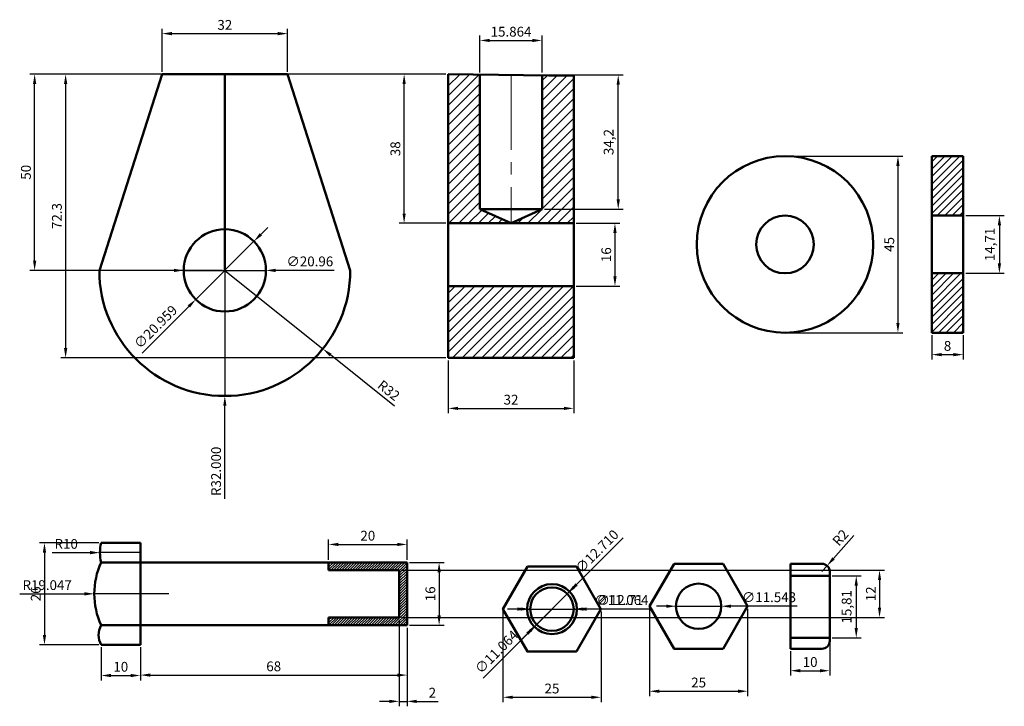
# Model space of a CAD drawing. Units: millimetres. Extents: x 1132 to 1696, y 1793 to 2376.
# Tile 1 of 4: x 1143 to 1394, y 1793 to 1968. Entities that reach past the tile are written whole.
import ezdxf

# ---------------------------------------------------------------- set-up
doc = ezdxf.new("R2010")
doc.units = ezdxf.units.MM
doc.linetypes.add('CENTER2', pattern=[28.575, 19.05, -3.175, 3.175, -3.175])
for name, color, linetype, lineweight in [('M-CNTR', 1, 'CENTER2', 18), ('M-DIMS', 2, 'Continuous', 25), ('M-HATC', 8, 'Continuous', 18), ('M-OUTL', 7, 'Continuous', 50)]:
    doc.layers.add(name, color=color, linetype=linetype, lineweight=lineweight)
doc.styles.get("Standard").update_dxf_attribs({"font": 'arial.ttf'})
doc.dimstyles.new('ISO-25', dxfattribs={"dimtxt": 2.5, "dimasz": 2.5, "dimexe": 1.25, "dimexo": 0.625, "dimtad": 1, "dimtxsty": 'Standard', "dimcen": 2.5, "dimadec": 0, "dimazin": 0, "dimtfac": 1, "dimtmove": 0, "dimatfit": 3, "dimfxl": 1, "dimarcsym": 0})

# ---------------------------------------------------------------- blocks, each defined once
blk = doc.blocks.new('*D15')
at = {"layer": 'Defpoints', "color": 0, "transparency": 16777216}
for p in [(1195.39, 1904.36), (1220.39, 1884.38)]:
    blk.add_point(p, dxfattribs=at)
at = {"layer": 'M-DIMS', "color": 0, "lineweight": -2, "transparency": 16777216}
for p, q in [((1195.39, 1904.36), (1220.39, 1884.38)), ((1238.63, 1869.8), (1222.34, 1882.82))]:
    blk.add_line(p, q, dxfattribs=at)
at = {"layer": 'M-DIMS', "color": 0, "transparency": 16777216}
blk.add_solid([(1222.6, 1883.14), (1222.08, 1882.49), (1220.39, 1884.38)], dxfattribs=at)
at = {"layer": 'M-DIMS', "color": 0, "transparency": 16777216, "insert": (1237.01, 1873.53), "char_height": 2.5, "attachment_point": 5, "rotation": 321.365}
blk.add_mtext('R32', dxfattribs=at)
blk = doc.blocks.new('*D16')
at = {"layer": 'Defpoints', "color": 0, "transparency": 16777216}
for p in [(1146.89, 1954.36), (1195.39, 1954.36), (1195.39, 1904.36)]:
    blk.add_point(p, dxfattribs=at)
at = {"layer": 'M-DIMS', "color": 0, "lineweight": -2, "transparency": 16777216}
for p, q in [((1194.77, 1954.36), (1145.64, 1954.36)), ((1146.89, 1906.86), (1146.89, 1951.86)), ((1194.77, 1904.36), (1145.64, 1904.36))]:
    blk.add_line(p, q, dxfattribs=at)
at = {"layer": 'M-DIMS', "color": 0, "transparency": 16777216}
for points in [[(1146.48, 1951.86), (1147.31, 1951.86), (1146.89, 1954.36)], [(1146.48, 1906.86), (1147.31, 1906.86), (1146.89, 1904.36)]]:
    blk.add_solid(points, dxfattribs=at)
at = {"layer": 'M-DIMS', "color": 0, "transparency": 16777216, "insert": (1144.99, 1929.36), "char_height": 2.5, "attachment_point": 5, "rotation": 90}
blk.add_mtext('50', dxfattribs=at)
blk = doc.blocks.new('*D17')
at = {"layer": 'Defpoints', "color": 0, "transparency": 16777216}
for p in [(1211.39, 1964.7), (1179.39, 1954.36), (1211.39, 1954.36)]:
    blk.add_point(p, dxfattribs=at)
at = {"layer": 'M-DIMS', "color": 0, "lineweight": -2, "transparency": 16777216}
for p, q in [((1179.39, 1954.98), (1179.39, 1965.95)), ((1181.89, 1964.7), (1208.89, 1964.7)), ((1211.39, 1954.98), (1211.39, 1965.95))]:
    blk.add_line(p, q, dxfattribs=at)
at = {"layer": 'M-DIMS', "color": 0, "transparency": 16777216}
for points in [[(1181.89, 1965.12), (1181.89, 1964.28), (1179.39, 1964.7)], [(1208.89, 1965.12), (1208.89, 1964.28), (1211.39, 1964.7)]]:
    blk.add_solid(points, dxfattribs=at)
at = {"layer": 'M-DIMS', "color": 0, "transparency": 16777216, "insert": (1195.39, 1966.6), "char_height": 2.5, "attachment_point": 5}
blk.add_mtext('32', dxfattribs=at)
blk = doc.blocks.new('*D18')
at = {"layer": 'Defpoints', "color": 0, "transparency": 16777216}
for p in [(1252.38, 1882.05), (1284.38, 1882.05), (1284.38, 1869.2)]:
    blk.add_point(p, dxfattribs=at)
at = {"layer": 'M-DIMS', "color": 0, "lineweight": -2, "transparency": 16777216}
for p, q in [((1252.38, 1881.43), (1252.38, 1867.95)), ((1284.38, 1881.43), (1284.38, 1867.95)), ((1254.88, 1869.2), (1281.88, 1869.2))]:
    blk.add_line(p, q, dxfattribs=at)
at = {"layer": 'M-DIMS', "color": 0, "transparency": 16777216}
for points in [[(1254.88, 1869.61), (1254.88, 1868.78), (1252.38, 1869.2)], [(1281.88, 1869.61), (1281.88, 1868.78), (1284.38, 1869.2)]]:
    blk.add_solid(points, dxfattribs=at)
at = {"layer": 'M-DIMS', "color": 0, "transparency": 16777216, "insert": (1268.38, 1871.1), "char_height": 2.5, "attachment_point": 5}
blk.add_mtext('32', dxfattribs=at)
blk = doc.blocks.new('*D19')
at = {"layer": 'Defpoints', "color": 0, "transparency": 16777216}
for p in [(1284.38, 1916.36), (1284.38, 1900.36), (1294.89, 1900.36)]:
    blk.add_point(p, dxfattribs=at)
at = {"layer": 'M-DIMS', "color": 0, "lineweight": -2, "transparency": 16777216}
for p, q in [((1285, 1916.36), (1296.14, 1916.36)), ((1294.89, 1913.86), (1294.89, 1902.86)), ((1285, 1900.36), (1296.14, 1900.36))]:
    blk.add_line(p, q, dxfattribs=at)
at = {"layer": 'M-DIMS', "color": 0, "transparency": 16777216}
for points in [[(1294.47, 1913.86), (1295.31, 1913.86), (1294.89, 1916.36)], [(1294.47, 1902.86), (1295.31, 1902.86), (1294.89, 1900.36)]]:
    blk.add_solid(points, dxfattribs=at)
at = {"layer": 'M-DIMS', "color": 0, "transparency": 16777216, "insert": (1292.99, 1908.36), "char_height": 2.5, "attachment_point": 5, "rotation": 90}
blk.add_mtext('16', dxfattribs=at)
blk = doc.blocks.new('*D20')
at = {"layer": 'Defpoints', "color": 0, "transparency": 16777216}
for p in [(1276.32, 1954.16), (1295.72, 1954.16), (1276.32, 1919.96)]:
    blk.add_point(p, dxfattribs=at)
at = {"layer": 'M-DIMS', "color": 0, "lineweight": -2, "transparency": 16777216}
for p, q in [((1276.94, 1954.16), (1296.97, 1954.16)), ((1295.72, 1922.46), (1295.72, 1951.66)), ((1276.94, 1919.96), (1296.97, 1919.96))]:
    blk.add_line(p, q, dxfattribs=at)
at = {"layer": 'M-DIMS', "color": 0, "transparency": 16777216}
for points in [[(1295.31, 1951.66), (1296.14, 1951.66), (1295.72, 1954.16)], [(1295.31, 1922.46), (1296.14, 1922.46), (1295.72, 1919.96)]]:
    blk.add_solid(points, dxfattribs=at)
at = {"layer": 'M-DIMS', "color": 0, "transparency": 16777216, "insert": (1293.6, 1937.06), "char_height": 2.5, "attachment_point": 5, "rotation": 90}
blk.add_mtext('34,2', dxfattribs=at)
blk = doc.blocks.new('*D21')
at = {"layer": 'Defpoints', "color": 0, "transparency": 16777216}
for p in [(1241.12, 1954.36), (1252.38, 1954.36), (1252.38, 1916.36)]:
    blk.add_point(p, dxfattribs=at)
at = {"layer": 'M-DIMS', "color": 0, "lineweight": -2, "transparency": 16777216}
for p, q in [((1251.75, 1954.36), (1239.87, 1954.36)), ((1241.12, 1918.86), (1241.12, 1951.86)), ((1251.75, 1916.36), (1239.87, 1916.36))]:
    blk.add_line(p, q, dxfattribs=at)
at = {"layer": 'M-DIMS', "color": 0, "transparency": 16777216}
for points in [[(1240.71, 1951.86), (1241.54, 1951.86), (1241.12, 1954.36)], [(1240.71, 1918.86), (1241.54, 1918.86), (1241.12, 1916.36)]]:
    blk.add_solid(points, dxfattribs=at)
at = {"layer": 'M-DIMS', "color": 0, "transparency": 16777216, "insert": (1239.22, 1935.36), "char_height": 2.5, "attachment_point": 5, "rotation": 90}
blk.add_mtext('38', dxfattribs=at)
blk = doc.blocks.new('*D22')
at = {"layer": 'Defpoints', "color": 0, "transparency": 16777216}
for p in [(1241.86, 1813.94), (1173.86, 1808.94), (1241.86, 1801.24)]:
    blk.add_point(p, dxfattribs=at)
at = {"layer": 'M-DIMS', "color": 0, "lineweight": -2, "transparency": 16777216}
for p, q in [((1241.86, 1813.32), (1241.86, 1799.99)), ((1173.86, 1808.32), (1173.86, 1799.99)), ((1176.36, 1801.24), (1239.36, 1801.24))]:
    blk.add_line(p, q, dxfattribs=at)
at = {"layer": 'M-DIMS', "color": 0, "transparency": 16777216}
for points in [[(1176.36, 1801.65), (1176.36, 1800.82), (1173.86, 1801.24)], [(1239.36, 1801.65), (1239.36, 1800.82), (1241.86, 1801.24)]]:
    blk.add_solid(points, dxfattribs=at)
at = {"layer": 'M-DIMS', "color": 0, "transparency": 16777216, "insert": (1207.86, 1803.14), "char_height": 2.5, "attachment_point": 5}
blk.add_mtext('68', dxfattribs=at)
blk = doc.blocks.new('*D23')
at = {"layer": 'Defpoints', "color": 0, "transparency": 16777216}
for p in [(1163.86, 1808.94), (1173.86, 1808.94), (1173.86, 1801.13)]:
    blk.add_point(p, dxfattribs=at)
at = {"layer": 'M-DIMS', "color": 0, "lineweight": -2, "transparency": 16777216}
for p, q in [((1163.86, 1808.32), (1163.86, 1799.88)), ((1173.86, 1808.32), (1173.86, 1799.88)), ((1166.36, 1801.13), (1171.36, 1801.13))]:
    blk.add_line(p, q, dxfattribs=at)
at = {"layer": 'M-DIMS', "color": 0, "transparency": 16777216}
for points in [[(1166.36, 1801.55), (1166.36, 1800.71), (1163.86, 1801.13)], [(1171.36, 1801.55), (1171.36, 1800.71), (1173.86, 1801.13)]]:
    blk.add_solid(points, dxfattribs=at)
at = {"layer": 'M-DIMS', "color": 0, "transparency": 16777216, "insert": (1168.86, 1803.03), "char_height": 2.5, "attachment_point": 5}
blk.add_mtext('10', dxfattribs=at)
blk = doc.blocks.new('*D24')
at = {"layer": 'Defpoints', "color": 0, "transparency": 16777216}
for p in [(1241.86, 1834.53), (1221.86, 1829.94), (1241.86, 1829.94)]:
    blk.add_point(p, dxfattribs=at)
at = {"layer": 'M-DIMS', "color": 0, "lineweight": -2, "transparency": 16777216}
for p, q in [((1221.86, 1830.57), (1221.86, 1835.78)), ((1241.86, 1830.57), (1241.86, 1835.78)), ((1224.36, 1834.53), (1239.36, 1834.53))]:
    blk.add_line(p, q, dxfattribs=at)
at = {"layer": 'M-DIMS', "color": 0, "transparency": 16777216}
for points in [[(1224.36, 1834.95), (1224.36, 1834.12), (1221.86, 1834.53)], [(1239.36, 1834.95), (1239.36, 1834.12), (1241.86, 1834.53)]]:
    blk.add_solid(points, dxfattribs=at)
at = {"layer": 'M-DIMS', "color": 0, "transparency": 16777216, "insert": (1231.86, 1836.43), "char_height": 2.5, "attachment_point": 5}
blk.add_mtext('20', dxfattribs=at)
blk = doc.blocks.new('*D25')
at = {"layer": 'Defpoints', "color": 0, "transparency": 16777216}
for p in [(1241.86, 1829.94), (1241.86, 1813.94), (1250.04, 1813.94)]:
    blk.add_point(p, dxfattribs=at)
at = {"layer": 'M-DIMS', "color": 0, "lineweight": -2, "transparency": 16777216}
for p, q in [((1242.49, 1829.94), (1251.29, 1829.94)), ((1250.04, 1827.44), (1250.04, 1816.44)), ((1242.49, 1813.94), (1251.29, 1813.94))]:
    blk.add_line(p, q, dxfattribs=at)
at = {"layer": 'M-DIMS', "color": 0, "transparency": 16777216}
for points in [[(1249.62, 1827.44), (1250.46, 1827.44), (1250.04, 1829.94)], [(1249.62, 1816.44), (1250.46, 1816.44), (1250.04, 1813.94)]]:
    blk.add_solid(points, dxfattribs=at)
at = {"layer": 'M-DIMS', "color": 0, "transparency": 16777216, "insert": (1248.14, 1821.94), "char_height": 2.5, "attachment_point": 5, "rotation": 90}
blk.add_mtext('16', dxfattribs=at)
blk = doc.blocks.new('*D26')
at = {"layer": 'Defpoints', "color": 0, "transparency": 16777216}
for p in [(1266.33, 1818.06), (1291.33, 1818.06), (1291.33, 1795.59)]:
    blk.add_point(p, dxfattribs=at)
at = {"layer": 'M-DIMS', "color": 0, "lineweight": -2, "transparency": 16777216}
for p, q in [((1266.33, 1817.44), (1266.33, 1794.34)), ((1291.33, 1817.44), (1291.33, 1794.34)), ((1268.83, 1795.59), (1288.83, 1795.59))]:
    blk.add_line(p, q, dxfattribs=at)
at = {"layer": 'M-DIMS', "color": 0, "transparency": 16777216}
for points in [[(1268.83, 1796), (1268.83, 1795.17), (1266.33, 1795.59)], [(1288.83, 1796), (1288.83, 1795.17), (1291.33, 1795.59)]]:
    blk.add_solid(points, dxfattribs=at)
at = {"layer": 'M-DIMS', "color": 0, "transparency": 16777216, "insert": (1278.83, 1797.49), "char_height": 2.5, "attachment_point": 5}
blk.add_mtext('25', dxfattribs=at)
blk = doc.blocks.new('*D27')
at = {"layer": 'Defpoints', "color": 0, "transparency": 16777216}
for p in [(1303.73, 1818.79), (1328.73, 1818.79), (1328.73, 1797.12)]:
    blk.add_point(p, dxfattribs=at)
at = {"layer": 'M-DIMS', "color": 0, "lineweight": -2, "transparency": 16777216}
for p, q in [((1303.73, 1818.16), (1303.73, 1795.87)), ((1328.73, 1818.16), (1328.73, 1795.87)), ((1306.23, 1797.12), (1326.23, 1797.12))]:
    blk.add_line(p, q, dxfattribs=at)
at = {"layer": 'M-DIMS', "color": 0, "transparency": 16777216}
for points in [[(1306.23, 1797.54), (1306.23, 1796.7), (1303.73, 1797.12)], [(1326.23, 1797.54), (1326.23, 1796.7), (1328.73, 1797.12)]]:
    blk.add_solid(points, dxfattribs=at)
at = {"layer": 'M-DIMS', "color": 0, "transparency": 16777216, "insert": (1316.23, 1799.02), "char_height": 2.5, "attachment_point": 5}
blk.add_mtext('25', dxfattribs=at)
blk = doc.blocks.new('*D28')
at = {"layer": 'Defpoints', "color": 0, "transparency": 16777216}
for p in [(1349.66, 1810.75), (1339.66, 1807.96), (1349.66, 1802.35)]:
    blk.add_point(p, dxfattribs=at)
at = {"layer": 'M-DIMS', "color": 0, "lineweight": -2, "transparency": 16777216}
for p, q in [((1349.66, 1810.12), (1349.66, 1801.1)), ((1339.66, 1807.34), (1339.66, 1801.1)), ((1342.16, 1802.35), (1347.16, 1802.35))]:
    blk.add_line(p, q, dxfattribs=at)
at = {"layer": 'M-DIMS', "color": 0, "transparency": 16777216}
for points in [[(1342.16, 1802.77), (1342.16, 1801.94), (1339.66, 1802.35)], [(1347.16, 1802.77), (1347.16, 1801.94), (1349.66, 1802.35)]]:
    blk.add_solid(points, dxfattribs=at)
at = {"layer": 'M-DIMS', "color": 0, "transparency": 16777216, "insert": (1344.66, 1804.25), "char_height": 2.5, "attachment_point": 5}
blk.add_mtext('10', dxfattribs=at)
blk = doc.blocks.new('*D29')
at = {"layer": 'Defpoints', "color": 0, "transparency": 16777216}
for p in [(1349.66, 1826.55), (1349.66, 1810.75), (1356.42, 1810.75)]:
    blk.add_point(p, dxfattribs=at)
at = {"layer": 'M-DIMS', "color": 0, "lineweight": -2, "transparency": 16777216}
for p, q in [((1350.29, 1826.55), (1357.67, 1826.55)), ((1356.42, 1824.05), (1356.42, 1813.25)), ((1350.29, 1810.75), (1357.67, 1810.75))]:
    blk.add_line(p, q, dxfattribs=at)
at = {"layer": 'M-DIMS', "color": 0, "transparency": 16777216}
for points in [[(1356.01, 1824.05), (1356.84, 1824.05), (1356.42, 1826.55)], [(1356.01, 1813.25), (1356.84, 1813.25), (1356.42, 1810.75)]]:
    blk.add_solid(points, dxfattribs=at)
at = {"layer": 'M-DIMS', "color": 0, "transparency": 16777216, "insert": (1354.29, 1818.65), "char_height": 2.5, "attachment_point": 5, "rotation": 90}
blk.add_mtext('15,81', dxfattribs=at)
blk = doc.blocks.new('*D30')
at = {"layer": 'Defpoints', "color": 0, "transparency": 16777216}
for p in [(1338.27, 1933.48), (1338.27, 1888.48), (1367.06, 1888.48)]:
    blk.add_point(p, dxfattribs=at)
at = {"layer": 'M-DIMS', "color": 0, "lineweight": -2, "transparency": 16777216}
for p, q in [((1338.9, 1933.48), (1368.31, 1933.48)), ((1367.06, 1930.98), (1367.06, 1890.98)), ((1338.9, 1888.48), (1368.31, 1888.48))]:
    blk.add_line(p, q, dxfattribs=at)
at = {"layer": 'M-DIMS', "color": 0, "transparency": 16777216}
for points in [[(1366.64, 1930.98), (1367.47, 1930.98), (1367.06, 1933.48)], [(1366.64, 1890.98), (1367.47, 1890.98), (1367.06, 1888.48)]]:
    blk.add_solid(points, dxfattribs=at)
at = {"layer": 'M-DIMS', "color": 0, "transparency": 16777216, "insert": (1365.16, 1910.98), "char_height": 2.5, "attachment_point": 5, "rotation": 90}
blk.add_mtext('45', dxfattribs=at)
blk = doc.blocks.new('*D31')
at = {"layer": 'Defpoints', "color": 0, "transparency": 16777216}
for p in [(1375.71, 1888.48), (1383.71, 1888.48), (1383.71, 1882.89)]:
    blk.add_point(p, dxfattribs=at)
at = {"layer": 'M-DIMS', "color": 0, "lineweight": -2, "transparency": 16777216}
for p, q in [((1375.71, 1887.85), (1375.71, 1881.64)), ((1383.71, 1887.85), (1383.71, 1881.64)), ((1378.21, 1882.89), (1381.21, 1882.89))]:
    blk.add_line(p, q, dxfattribs=at)
at = {"layer": 'M-DIMS', "color": 0, "transparency": 16777216}
for points in [[(1378.21, 1883.31), (1378.21, 1882.48), (1375.71, 1882.89)], [(1381.21, 1883.31), (1381.21, 1882.48), (1383.71, 1882.89)]]:
    blk.add_solid(points, dxfattribs=at)
at = {"layer": 'M-DIMS', "color": 0, "transparency": 16777216, "insert": (1379.71, 1884.8), "char_height": 2.5, "attachment_point": 5}
blk.add_mtext('8', dxfattribs=at)
blk = doc.blocks.new('*D32')
at = {"layer": 'Defpoints', "color": 0, "transparency": 16777216}
for p in [(1383.71, 1918.33), (1383.71, 1903.62), (1392.93, 1903.62)]:
    blk.add_point(p, dxfattribs=at)
at = {"layer": 'M-DIMS', "color": 0, "lineweight": -2, "transparency": 16777216}
for p, q in [((1384.33, 1918.33), (1394.18, 1918.33)), ((1392.93, 1915.83), (1392.93, 1906.12)), ((1384.33, 1903.62), (1394.18, 1903.62))]:
    blk.add_line(p, q, dxfattribs=at)
at = {"layer": 'M-DIMS', "color": 0, "transparency": 16777216}
for points in [[(1392.52, 1915.83), (1393.35, 1915.83), (1392.93, 1918.33)], [(1392.52, 1906.12), (1393.35, 1906.12), (1392.93, 1903.62)]]:
    blk.add_solid(points, dxfattribs=at)
at = {"layer": 'M-DIMS', "color": 0, "transparency": 16777216, "insert": (1390.81, 1910.98), "char_height": 2.5, "attachment_point": 5, "rotation": 90}
blk.add_mtext('14,71', dxfattribs=at)
blk = doc.blocks.new('*D39')
at = {"layer": 'Defpoints', "color": 0, "transparency": 16777216}
for p in [(1276.32, 1962.96), (1260.45, 1954.16), (1276.32, 1954.16)]:
    blk.add_point(p, dxfattribs=at)
at = {"layer": 'M-DIMS', "color": 0, "lineweight": -2, "transparency": 16777216}
for p, q in [((1260.45, 1954.78), (1260.45, 1964.21)), ((1276.32, 1954.78), (1276.32, 1964.21)), ((1262.95, 1962.96), (1273.82, 1962.96))]:
    blk.add_line(p, q, dxfattribs=at)
at = {"layer": 'M-DIMS', "color": 0, "transparency": 16777216}
for points in [[(1262.95, 1963.37), (1262.95, 1962.54), (1260.45, 1962.96)], [(1273.82, 1963.37), (1273.82, 1962.54), (1276.32, 1962.96)]]:
    blk.add_solid(points, dxfattribs=at)
at = {"layer": 'M-DIMS', "color": 0, "transparency": 16777216, "insert": (1268.39, 1964.86), "char_height": 2.5, "attachment_point": 5}
blk.add_mtext('15.864', dxfattribs=at)
blk = doc.blocks.new('*D40')
at = {"layer": 'Defpoints', "color": 0, "transparency": 16777216}
for p in [(1252.38, 1954.36), (1154.79, 1882.05), (1252.38, 1882.05)]:
    blk.add_point(p, dxfattribs=at)
at = {"layer": 'M-DIMS', "color": 0, "lineweight": -2, "transparency": 16777216}
for p, q in [((1251.75, 1954.36), (1153.54, 1954.36)), ((1154.79, 1951.86), (1154.79, 1884.55)), ((1251.75, 1882.05), (1153.54, 1882.05))]:
    blk.add_line(p, q, dxfattribs=at)
at = {"layer": 'M-DIMS', "color": 0, "transparency": 16777216}
for points in [[(1154.38, 1951.86), (1155.21, 1951.86), (1154.79, 1954.36)], [(1154.38, 1884.55), (1155.21, 1884.55), (1154.79, 1882.05)]]:
    blk.add_solid(points, dxfattribs=at)
at = {"layer": 'M-DIMS', "color": 0, "transparency": 16777216, "insert": (1152.89, 1918.21), "char_height": 2.5, "attachment_point": 5, "rotation": 90}
blk.add_mtext('72.3', dxfattribs=at)
blk = doc.blocks.new('*D46')
at = {"layer": 'Defpoints', "color": 0, "transparency": 16777216}
for p in [(1163.86, 1834.94), (1149.4, 1808.94), (1163.86, 1808.94)]:
    blk.add_point(p, dxfattribs=at)
at = {"layer": 'M-DIMS', "color": 0, "lineweight": -2, "transparency": 16777216}
for p, q in [((1163.24, 1834.94), (1148.15, 1834.94)), ((1149.4, 1832.44), (1149.4, 1811.44)), ((1163.24, 1808.94), (1148.15, 1808.94))]:
    blk.add_line(p, q, dxfattribs=at)
at = {"layer": 'M-DIMS', "color": 0, "transparency": 16777216}
for points in [[(1148.98, 1832.44), (1149.82, 1832.44), (1149.4, 1834.94)], [(1148.98, 1811.44), (1149.82, 1811.44), (1149.4, 1808.94)]]:
    blk.add_solid(points, dxfattribs=at)
at = {"layer": 'M-DIMS', "color": 0, "transparency": 16777216, "insert": (1147.5, 1821.94), "char_height": 2.5, "attachment_point": 5, "rotation": 90}
blk.add_mtext('26', dxfattribs=at)
blk = doc.blocks.new('*D47')
at = {"layer": 'Defpoints', "color": 0, "transparency": 16777216}
for p in [(1239.86, 1827.94), (1239.86, 1815.94), (1362.36, 1815.94)]:
    blk.add_point(p, dxfattribs=at)
at = {"layer": 'M-DIMS', "color": 0, "lineweight": -2, "transparency": 16777216}
for p, q in [((1240.49, 1827.94), (1363.61, 1827.94)), ((1362.36, 1825.44), (1362.36, 1818.44)), ((1240.49, 1815.94), (1363.61, 1815.94))]:
    blk.add_line(p, q, dxfattribs=at)
at = {"layer": 'M-DIMS', "color": 0, "transparency": 16777216}
for points in [[(1361.95, 1825.44), (1362.78, 1825.44), (1362.36, 1827.94)], [(1361.95, 1818.44), (1362.78, 1818.44), (1362.36, 1815.94)]]:
    blk.add_solid(points, dxfattribs=at)
at = {"layer": 'M-DIMS', "color": 0, "transparency": 16777216, "insert": (1360.48, 1821.94), "char_height": 2.5, "attachment_point": 5, "rotation": 90}
blk.add_mtext('12', dxfattribs=at)
blk = doc.blocks.new('*D48')
at = {"layer": 'Defpoints', "color": 0, "transparency": 16777216}
for p in [(1239.86, 1815.94), (1241.86, 1813.94), (1241.86, 1794.54)]:
    blk.add_point(p, dxfattribs=at)
at = {"layer": 'M-DIMS', "color": 0, "lineweight": -2, "transparency": 16777216}
for p, q in [((1239.86, 1815.32), (1239.86, 1793.29)), ((1241.86, 1813.32), (1241.86, 1793.29)), ((1237.36, 1794.54), (1234.86, 1794.54)), ((1239.86, 1794.54), (1241.86, 1794.54)), ((1244.36, 1794.54), (1249.77, 1794.54))]:
    blk.add_line(p, q, dxfattribs=at)
at = {"layer": 'M-DIMS', "color": 0, "transparency": 16777216}
for points in [[(1237.36, 1794.95), (1237.36, 1794.12), (1239.86, 1794.54)], [(1244.36, 1794.95), (1244.36, 1794.12), (1241.86, 1794.54)]]:
    blk.add_solid(points, dxfattribs=at)
at = {"layer": 'M-DIMS', "color": 0, "transparency": 16777216, "insert": (1248.32, 1796.42), "char_height": 2.5, "attachment_point": 5}
blk.add_mtext('2', dxfattribs=at)
blk = doc.blocks.new('*D50')
at = {"layer": 'Defpoints', "color": 0, "transparency": 16777216}
for p in [(1184.91, 1904.36), (1205.87, 1904.36)]:
    blk.add_point(p, dxfattribs=at)
at = {"layer": 'M-DIMS', "color": 0, "lineweight": -2, "transparency": 16777216}
for p, q in [((1182.41, 1904.36), (1179.91, 1904.36)), ((1184.91, 1904.36), (1205.87, 1904.36)), ((1223.28, 1904.36), (1208.37, 1904.36))]:
    blk.add_line(p, q, dxfattribs=at)
at = {"layer": 'M-DIMS', "color": 0, "transparency": 16777216}
for points in [[(1182.41, 1904.78), (1182.41, 1903.94), (1184.91, 1904.36)], [(1208.37, 1904.77), (1208.37, 1903.94), (1205.87, 1904.36)]]:
    blk.add_solid(points, dxfattribs=at)
at = {"layer": 'M-DIMS', "color": 0, "transparency": 16777216, "insert": (1217.08, 1906.33), "char_height": 2.5, "attachment_point": 5, "rotation": 359.9985}
blk.add_mtext('∅20.96', dxfattribs=at)
blk = doc.blocks.new('*D54')
at = {"layer": 'Defpoints', "color": 0, "transparency": 16777216}
for p in [(1162.1, 1821.94), (1181.15, 1821.94)]:
    blk.add_point(p, dxfattribs=at)
at = {"layer": 'M-DIMS', "color": 0, "lineweight": -2, "transparency": 16777216}
for p, q in [((1143.08, 1821.94), (1159.6, 1821.94)), ((1181.15, 1821.94), (1162.1, 1821.94))]:
    blk.add_line(p, q, dxfattribs=at)
at = {"layer": 'M-DIMS', "color": 0, "transparency": 16777216}
blk.add_solid([(1159.6, 1822.36), (1159.6, 1821.53), (1162.1, 1821.94)], dxfattribs=at)
at = {"layer": 'M-DIMS', "color": 0, "transparency": 16777216, "insert": (1150.09, 1823.84), "char_height": 2.5, "attachment_point": 5, "rotation": 0.0015}
blk.add_mtext('R19.047', dxfattribs=at)
blk = doc.blocks.new('*D55')
at = {"layer": 'Defpoints', "color": 0, "transparency": 16777216}
for p in [(1163.55, 1832.44), (1173.55, 1832.44)]:
    blk.add_point(p, dxfattribs=at)
at = {"layer": 'M-DIMS', "color": 0, "lineweight": -2, "transparency": 16777216}
for p, q in [((1151.33, 1832.44), (1161.05, 1832.44)), ((1173.55, 1832.44), (1163.55, 1832.44))]:
    blk.add_line(p, q, dxfattribs=at)
at = {"layer": 'M-DIMS', "color": 0, "transparency": 16777216}
blk.add_solid([(1161.05, 1832.86), (1161.05, 1832.03), (1163.55, 1832.44)], dxfattribs=at)
at = {"layer": 'M-DIMS', "color": 0, "transparency": 16777216, "insert": (1154.94, 1834.34), "char_height": 2.5, "attachment_point": 5, "rotation": 0.0028}
blk.add_mtext('R10', dxfattribs=at)
blk = doc.blocks.new('*D56')
at = {"layer": 'Defpoints', "color": 0, "transparency": 16777216}
for p in [(1272.47, 1818.06), (1285.18, 1818.06)]:
    blk.add_point(p, dxfattribs=at)
at = {"layer": 'M-DIMS', "color": 0, "lineweight": -2, "transparency": 16777216}
for p, q in [((1269.97, 1818.06), (1267.47, 1818.06)), ((1272.47, 1818.06), (1285.18, 1818.06)), ((1302.11, 1818.06), (1287.68, 1818.06))]:
    blk.add_line(p, q, dxfattribs=at)
at = {"layer": 'M-DIMS', "color": 0, "transparency": 16777216}
for points in [[(1269.97, 1818.48), (1269.97, 1817.65), (1272.47, 1818.06)], [(1287.68, 1818.48), (1287.68, 1817.64), (1285.18, 1818.06)]]:
    blk.add_solid(points, dxfattribs=at)
at = {"layer": 'M-DIMS', "color": 0, "transparency": 16777216, "insert": (1296.15, 1820.03), "char_height": 2.5, "attachment_point": 5, "rotation": 359.9964}
blk.add_mtext('∅12.71', dxfattribs=at)
blk = doc.blocks.new('*D57')
at = {"layer": 'Defpoints', "color": 0, "transparency": 16777216}
for p in [(1273.3, 1818.06), (1284.36, 1818.06)]:
    blk.add_point(p, dxfattribs=at)
at = {"layer": 'M-DIMS', "color": 0, "lineweight": -2, "transparency": 16777216}
for p, q in [((1270.8, 1818.06), (1268.3, 1818.06)), ((1273.3, 1818.06), (1284.36, 1818.06)), ((1303.7, 1818.06), (1286.86, 1818.06))]:
    blk.add_line(p, q, dxfattribs=at)
at = {"layer": 'M-DIMS', "color": 0, "transparency": 16777216}
for points in [[(1270.8, 1818.48), (1270.8, 1817.65), (1273.3, 1818.06)], [(1286.86, 1818.48), (1286.86, 1817.64), (1284.36, 1818.06)]]:
    blk.add_solid(points, dxfattribs=at)
at = {"layer": 'M-DIMS', "color": 0, "transparency": 16777216, "insert": (1296.53, 1820.03), "char_height": 2.5, "attachment_point": 5, "rotation": 359.9959}
blk.add_mtext('∅11.064', dxfattribs=at)
blk = doc.blocks.new('*D58')
at = {"layer": 'Defpoints', "color": 0, "transparency": 16777216}
for p in [(1310.46, 1818.79), (1322, 1818.79)]:
    blk.add_point(p, dxfattribs=at)
at = {"layer": 'M-DIMS', "color": 0, "lineweight": -2, "transparency": 16777216}
for p, q in [((1307.96, 1818.79), (1305.46, 1818.79)), ((1310.46, 1818.79), (1322, 1818.79)), ((1341.35, 1818.78), (1324.5, 1818.79))]:
    blk.add_line(p, q, dxfattribs=at)
at = {"layer": 'M-DIMS', "color": 0, "transparency": 16777216}
for points in [[(1307.96, 1819.2), (1307.96, 1818.37), (1310.46, 1818.79)], [(1324.5, 1819.2), (1324.5, 1818.37), (1322, 1818.79)]]:
    blk.add_solid(points, dxfattribs=at)
at = {"layer": 'M-DIMS', "color": 0, "transparency": 16777216, "insert": (1334.17, 1820.76), "char_height": 2.5, "attachment_point": 5, "rotation": 359.9969}
blk.add_mtext('∅11.543', dxfattribs=at)
blk = doc.blocks.new('*D59')
at = {"layer": 'Defpoints', "color": 0, "transparency": 16777216}
for p in [(1348.99, 1829.11), (1347.66, 1827.61)]:
    blk.add_point(p, dxfattribs=at)
at = {"layer": 'M-DIMS', "color": 0, "lineweight": -2, "transparency": 16777216}
for p, q in [((1355.79, 1836.79), (1350.65, 1830.98)), ((1347.66, 1827.61), (1348.99, 1829.11))]:
    blk.add_line(p, q, dxfattribs=at)
at = {"layer": 'M-DIMS', "color": 0, "transparency": 16777216}
blk.add_solid([(1350.33, 1831.26), (1350.96, 1830.7), (1348.99, 1829.11)], dxfattribs=at)
at = {"layer": 'M-DIMS', "color": 0, "transparency": 16777216, "insert": (1352.64, 1836.07), "char_height": 2.5, "attachment_point": 5, "rotation": 48.4719}
blk.add_mtext('R2', dxfattribs=at)
blk = doc.blocks.new('*D86')
at = {"layer": 'Defpoints', "color": 0, "transparency": 16777216}
for p in [(1202.81, 1911.77), (1187.98, 1896.95)]:
    blk.add_point(p, dxfattribs=at)
at = {"layer": 'M-DIMS', "color": 0, "lineweight": -2, "transparency": 16777216}
for p, q in [((1204.57, 1913.53), (1206.34, 1915.3)), ((1202.81, 1911.77), (1187.98, 1896.95)), ((1174.29, 1883.27), (1186.21, 1895.18))]:
    blk.add_line(p, q, dxfattribs=at)
at = {"layer": 'M-DIMS', "color": 0, "transparency": 16777216}
for points in [[(1204.28, 1913.83), (1204.87, 1913.24), (1202.81, 1911.77)], [(1185.92, 1895.48), (1186.51, 1894.89), (1187.98, 1896.95)]]:
    blk.add_solid(points, dxfattribs=at)
at = {"layer": 'M-DIMS', "color": 0, "transparency": 16777216, "insert": (1177.97, 1889.74), "char_height": 2.5, "attachment_point": 5, "rotation": 44.9813}
blk.add_mtext('∅20.959', dxfattribs=at)
blk = doc.blocks.new('*D87')
at = {"layer": 'Defpoints', "color": 0, "transparency": 16777216}
for p in [(1195.39, 1904.36), (1195.39, 1872.36)]:
    blk.add_point(p, dxfattribs=at)
at = {"layer": 'M-DIMS', "color": 0, "lineweight": -2, "transparency": 16777216}
for p, q in [((1195.39, 1904.36), (1195.39, 1872.36)), ((1195.39, 1846.15), (1195.39, 1869.86))]:
    blk.add_line(p, q, dxfattribs=at)
at = {"layer": 'M-DIMS', "color": 0, "transparency": 16777216}
blk.add_solid([(1194.98, 1869.86), (1195.81, 1869.86), (1195.39, 1872.36)], dxfattribs=at)
at = {"layer": 'M-DIMS', "color": 0, "transparency": 16777216, "insert": (1193.49, 1853.16), "char_height": 2.5, "attachment_point": 5, "rotation": 89.9998}
blk.add_mtext('R32.000', dxfattribs=at)
blk = doc.blocks.new('*D88')
at = {"layer": 'Defpoints', "color": 0, "transparency": 16777216}
for p in [(1283.32, 1822.55), (1274.33, 1813.57)]:
    blk.add_point(p, dxfattribs=at)
at = {"layer": 'M-DIMS', "color": 0, "lineweight": -2, "transparency": 16777216}
for p, q in [((1297, 1836.23), (1285.09, 1824.32)), ((1274.33, 1813.57), (1283.32, 1822.55)), ((1272.57, 1811.8), (1270.8, 1810.03))]:
    blk.add_line(p, q, dxfattribs=at)
at = {"layer": 'M-DIMS', "color": 0, "transparency": 16777216}
for points in [[(1284.8, 1824.62), (1285.39, 1824.03), (1283.32, 1822.55)], [(1272.27, 1812.1), (1272.86, 1811.51), (1274.33, 1813.57)]]:
    blk.add_solid(points, dxfattribs=at)
at = {"layer": 'M-DIMS', "color": 0, "transparency": 16777216, "insert": (1290.54, 1832.55), "char_height": 2.5, "attachment_point": 5, "rotation": 44.983}
blk.add_mtext('∅12.710', dxfattribs=at)
blk = doc.blocks.new('*D89')
at = {"layer": 'Defpoints', "color": 0, "transparency": 16777216}
for p in [(1282.74, 1821.97), (1274.92, 1814.15)]:
    blk.add_point(p, dxfattribs=at)
at = {"layer": 'M-DIMS', "color": 0, "lineweight": -2, "transparency": 16777216}
for p, q in [((1284.51, 1823.74), (1286.27, 1825.51)), ((1282.74, 1821.97), (1274.92, 1814.15)), ((1261.25, 1800.47), (1273.15, 1812.38))]:
    blk.add_line(p, q, dxfattribs=at)
at = {"layer": 'M-DIMS', "color": 0, "transparency": 16777216}
for points in [[(1284.21, 1824.04), (1284.8, 1823.45), (1282.74, 1821.97)], [(1272.86, 1812.67), (1273.45, 1812.09), (1274.92, 1814.15)]]:
    blk.add_solid(points, dxfattribs=at)
at = {"layer": 'M-DIMS', "color": 0, "transparency": 16777216, "insert": (1264.92, 1806.93), "char_height": 2.5, "attachment_point": 5, "rotation": 45.0195}
blk.add_mtext('∅11.064', dxfattribs=at)

msp = doc.modelspace()

# ---------------------------------------------------------------- hatches: boundary and pattern name
at = {"layer": 'M-HATC'}
h = msp.add_hatch(dxfattribs=at)
h.set_pattern_fill('ANSI31', color=256, scale=0.56)
h.paths.add_polyline_path([(1284.3772, 1953.9602), (1276.3177, 1954.0604), (1276.3177, 1919.9602), (1268.3772, 1916.3583), (1284.3772, 1916.3583)])
h.paths.add_polyline_path([(1260.4541, 1919.9602), (1260.4541, 1954.2578), (1252.3772, 1954.3583), (1252.3772, 1916.3583), (1268.3772, 1916.3583)])
h.paths.add_polyline_path([(1284.3772, 1900.3583), (1252.3772, 1900.3583), (1252.3772, 1882.0542), (1284.3772, 1882.0542)])
h = msp.add_hatch(dxfattribs=at)
h.set_pattern_fill('ANSI31', color=256, scale=0.42)
h.paths.add_polyline_path([(1383.7067, 1933.4789), (1375.7067, 1933.4789), (1375.7067, 1918.3333), (1383.7067, 1918.3333)])
h.paths.add_polyline_path([(1383.7067, 1903.6246), (1375.7067, 1903.6246), (1375.7067, 1888.4789), (1383.7067, 1888.4789)])
h = msp.add_hatch(dxfattribs=at)
h.set_pattern_fill('ANSI31', color=256, scale=0.15)
h.paths.add_polyline_path([(1241.8628, 1829.9425), (1221.8628, 1829.9425), (1221.8628, 1827.9425), (1239.8628, 1827.9425), (1239.8628, 1815.9425), (1221.8628, 1815.9425), (1221.8628, 1813.9425), (1241.8628, 1813.9425)])

# ---------------------------------------------------------------- linework, layer by layer
at = {"layer": 'M-CNTR'}
msp.add_line((1268.3772, 1954.1592), (1268.3772, 1916.3583), dxfattribs=at)
at = {"layer": 'M-OUTL'}
for p, q in [((1163.3931, 1904.3583), (1179.3931, 1954.3583)), ((1179.3931, 1954.3583), (1211.3931, 1954.3583)), ((1195.3931, 1954.3583), (1195.3931, 1904.3583)), ((1211.3931, 1954.3583), (1227.3931, 1904.3583)), ((1252.3772, 1954.3583), (1252.3772, 1882.0542)), ((1284.3772, 1953.9602), (1252.3772, 1954.3583)), ((1252.3772, 1954.3583), (1252.3772, 1916.3583)), ((1260.4541, 1954.1592), (1260.4541, 1919.9602)), ((1276.3177, 1954.1592), (1276.3177, 1919.9602)), ((1284.3772, 1882.0542), (1284.3772, 1953.9602)), ((1284.3772, 1953.9602), (1284.3772, 1919.9602)), ((1375.7067, 1933.4789), (1375.7067, 1888.4789)), ((1383.7067, 1933.4789), (1375.7067, 1933.4789)), ((1383.7067, 1888.4789), (1383.7067, 1933.4789)), ((1276.3177, 1919.9602), (1260.4541, 1919.9602)), ((1260.4541, 1919.9602), (1268.3772, 1916.3583)), ((1268.3772, 1916.3583), (1276.3177, 1919.9602)), ((1252.3772, 1916.3583), (1284.3772, 1916.3583)), ((1375.7067, 1918.3333), (1383.7067, 1918.3333)), ((1375.7067, 1903.6246), (1383.7067, 1903.6246)), ((1284.3772, 1900.3583), (1252.3772, 1900.3583)), ((1375.7067, 1888.4789), (1383.7067, 1888.4789)), ((1252.3772, 1882.0542), (1284.3772, 1882.0542)), ((1173.8628, 1834.9425), (1163.8628, 1834.9425)), ((1173.8628, 1829.9425), (1173.8628, 1834.9425)), ((1173.8628, 1829.9425), (1163.8628, 1829.9425)), ((1173.8628, 1829.9425), (1241.8628, 1829.9425)), ((1173.8628, 1813.9425), (1173.8628, 1829.9425)), ((1241.8628, 1829.9425), (1221.8628, 1829.9425)), ((1221.8628, 1829.9425), (1221.8628, 1827.9425)), ((1241.8628, 1829.9425), (1241.8628, 1813.9425)), ((1339.662, 1829.6116), (1339.662, 1807.961)), ((1339.662, 1829.6116), (1347.662, 1829.6116)), ((1221.8628, 1827.9425), (1239.8628, 1827.9425)), ((1239.8628, 1827.9425), (1239.8628, 1815.9425)), ((1339.662, 1826.5548), (1349.662, 1826.5548)), ((1349.662, 1809.961), (1349.662, 1827.6116)), ((1239.8628, 1815.9425), (1221.8628, 1815.9425)), ((1221.8628, 1815.9425), (1221.8628, 1813.9425)), ((1173.8628, 1813.9425), (1163.8628, 1813.9425)), ((1241.8628, 1813.9425), (1173.8628, 1813.9425)), ((1173.8628, 1808.9425), (1173.8628, 1813.9425)), ((1339.662, 1810.7467), (1349.662, 1810.7467)), ((1163.8628, 1808.9425), (1173.8628, 1808.9425)), ((1339.662, 1807.961), (1347.662, 1807.961))]:
    msp.add_line(p, q, dxfattribs=at)
for points in [[(1272.5787, 1828.8867), (1266.3287, 1818.0614), (1272.5787, 1807.2361), (1285.0787, 1807.2361), (1291.3287, 1818.0614), (1285.0787, 1828.8867)], [(1309.9765, 1829.6116), (1303.7265, 1818.7863), (1309.9765, 1807.961), (1322.4765, 1807.961), (1328.7265, 1818.7863), (1322.4765, 1829.6116)]]:
    msp.add_lwpolyline(points, close=True, dxfattribs=at)
for centre, radius in [((1338.2703, 1910.9789), 22.5), ((1338.2703, 1910.9789), 7.3543), ((1195.3931, 1904.3583), 10.4797), ((1278.8287, 1818.0614), 6.3549), ((1278.8287, 1818.0614), 5.5322), ((1316.2265, 1818.7863), 5.7714)]:
    msp.add_circle(centre, radius, dxfattribs=at)
for centre, radius, start, end in [((1195.3931, 1904.3583), 32, 180, 0), ((1173.5452, 1832.4425), 10, 165.522488, 194.477512), ((1181.1487, 1821.9425), 19.0474, 155.165061, 204.834939), ((1347.662, 1827.6116), 2, 360, 90), ((1168.1929, 1811.4425), 5, 150, 210), ((1347.662, 1809.961), 2, 270, 360)]:
    msp.add_arc(centre, radius, start, end, dxfattribs=at)

# ---------------------------------------------------------------- dimensions: what is measured, and where the dimension line sits
at = {"layer": 'M-DIMS'}
for base, p1, p2, override, picture, middle in [((1211.3931, 1964.7008), (1179.3931, 1954.3583), (1211.3931, 1954.3583), {"dimclrd": 0, "dimclre": 0, "dimclrt": 0}, '*D17', (1195.3931, 1966.6031)), ((1276.3177, 1962.9583), (1260.4541, 1954.1592), (1276.3177, 1954.1592), {"dimdec": 3, "dimlfac": 1, "dimrnd": 0, "dimzin": 0, "dimdsep": 46, "dimlunit": 2}, '*D39', (1268.3859, 1964.8597)), ((1383.7067, 1882.8936), (1375.7067, 1888.4789), (1383.7067, 1888.4789), {"dimclrd": 0, "dimclre": 0, "dimclrt": 0}, '*D31', (1379.7067, 1884.795)), ((1284.3772, 1869.1954), (1252.3772, 1882.0542), (1284.3772, 1882.0542), {"dimclrd": 0, "dimclre": 0, "dimclrt": 0}, '*D18', (1268.3772, 1871.0977)), ((1241.8628, 1834.5326), (1221.8628, 1829.9425), (1241.8628, 1829.9425), {"dimclrd": 0, "dimclre": 0, "dimclrt": 0}, '*D24', (1231.8628, 1836.434)), ((1291.3287, 1795.5869), (1266.3287, 1818.0614), (1291.3287, 1818.0614), {"dimclrd": 0, "dimclre": 0, "dimclrt": 0}, '*D26', (1278.8287, 1797.4884)), ((1328.7265, 1797.1187), (1303.7265, 1818.7863), (1328.7265, 1818.7863), {"dimclrd": 0, "dimclre": 0, "dimclrt": 0}, '*D27', (1316.2265, 1799.0202)), ((1241.8628, 1794.5361), (1239.8628, 1815.9425), (1241.8628, 1813.9425), {"dimdec": 0, "dimlfac": 1, "dimrnd": 0, "dimzin": 0, "dimdsep": 46, "dimlunit": 2}, '*D48', (1248.3157, 1796.4162)), ((1241.8628, 1801.2366), (1173.8628, 1808.9425), (1241.8628, 1813.9425), {"dimclrd": 0, "dimclre": 0, "dimclrt": 0}, '*D22', (1207.8628, 1803.138)), ((1349.662, 1802.3525), (1339.662, 1807.961), (1349.662, 1810.7467), {"dimclrd": 0, "dimclre": 0, "dimclrt": 0}, '*D28', (1344.662, 1804.2539)), ((1173.8628, 1801.1285), (1163.8628, 1808.9425), (1173.8628, 1808.9425), {"dimclrd": 0, "dimclre": 0, "dimclrt": 0}, '*D23', (1168.8628, 1803.03))]:
    dim = msp.add_linear_dim(base=base, p1=p1, p2=p2, dimstyle='ISO-25', override=override, dxfattribs=at)
    dim.commit()
    dim.dimension.update_dxf_attribs({"geometry": picture, "text_midpoint": middle})
for base, p1, p2, override, picture, middle in [((1146.894, 1954.3583), (1195.3931, 1904.3583), (1195.3931, 1954.3583), {"dimclrd": 0, "dimclre": 0, "dimclrt": 0}, '*D16', (1144.9926, 1929.3583)), ((1154.7931, 1882.0542), (1252.3772, 1954.3583), (1252.3772, 1882.0542), {"dimdec": 1, "dimlfac": 1, "dimrnd": 0, "dimzin": 0, "dimdsep": 46, "dimlunit": 2}, '*D40', (1152.8908, 1918.2062)), ((1241.1229, 1954.3583), (1252.3772, 1916.3583), (1252.3772, 1954.3583), {"dimclrd": 0, "dimclre": 0, "dimclrt": 0}, '*D21', (1239.2207, 1935.3583)), ((1295.7235, 1954.1592), (1276.3177, 1919.9602), (1276.3177, 1954.1592), {"dimclrd": 0, "dimclre": 0, "dimclrt": 0}, '*D20', (1293.5961, 1937.0597)), ((1367.056, 1888.4789), (1338.2703, 1933.4789), (1338.2703, 1888.4789), {"dimclrd": 0, "dimclre": 0, "dimclrt": 0}, '*D30', (1365.1597, 1910.9789)), ((1294.8894, 1900.3583), (1284.3772, 1916.3583), (1284.3772, 1900.3583), {"dimclrd": 0, "dimclre": 0, "dimclrt": 0}, '*D19', (1292.9879, 1908.3583)), ((1392.9328, 1903.6246), (1383.7067, 1918.3333), (1383.7067, 1903.6246), {"dimclrd": 0, "dimclre": 0, "dimclrt": 0}, '*D32', (1390.8054, 1910.9789)), ((1149.4013, 1808.9425), (1163.8628, 1834.9425), (1163.8628, 1808.9425), {"dimdec": 0, "dimlfac": 1, "dimrnd": 0, "dimzin": 0, "dimdsep": 46, "dimlunit": 2}, '*D46', (1147.4999, 1821.9425)), ((1250.0403, 1813.9425), (1241.8628, 1829.9425), (1241.8628, 1813.9425), {"dimclrd": 0, "dimclre": 0, "dimclrt": 0}, '*D25', (1248.1389, 1821.9425)), ((1362.362, 1815.9425), (1239.8628, 1827.9425), (1239.8628, 1815.9425), {"dimdec": 0, "dimlfac": 1, "dimrnd": 0, "dimzin": 0, "dimdsep": 46, "dimlunit": 2}, '*D47', (1360.4819, 1821.9425)), ((1356.4223, 1810.7467), (1349.662, 1826.5548), (1349.662, 1810.7467), {"dimclrd": 0, "dimclre": 0, "dimclrt": 0}, '*D29', (1354.2949, 1818.6507))]:
    dim = msp.add_linear_dim(base=base, p1=p1, p2=p2, angle=90, dimstyle='ISO-25', override=override, dxfattribs=at)
    dim.commit()
    dim.dimension.update_dxf_attribs({"geometry": picture, "text_midpoint": middle})
for p1, p2, override, picture, middle in [((1202.8058, 1911.7661), (1187.9804, 1896.9504), {"dimdec": 3, "dimlfac": 1, "dimrnd": 0, "dimzin": 0, "dimdsep": 46, "dimlunit": 2}, '*D86', (1179.3673, 1888.3429)), ((1184.9134, 1904.3585), (1205.8728, 1904.358), {"dimdec": 2, "dimlfac": 1, "dimrnd": 0, "dimzin": 0, "dimdsep": 46, "dimlunit": 2}, '*D50', (1217.075, 1904.3577)), ((1310.4551, 1818.7866), (1321.9979, 1818.786), {"dimdec": 3, "dimlfac": 1, "dimrnd": 0, "dimzin": 0, "dimdsep": 46, "dimlunit": 2}, '*D58', (1334.1722, 1818.7853))]:
    dim = msp.add_diameter_dim_2p(p1=p1, p2=p2, dimstyle='ISO-25', override=override, dxfattribs=at)
    dim.commit()
    dim.dimension.update_dxf_attribs({"geometry": picture, "text_midpoint": middle})
for mpoint, override, picture, middle in [((1195.393, 1872.3583), {"dimdec": 3, "dimlfac": 1, "dimrnd": 0, "dimzin": 0, "dimdsep": 46, "dimlunit": 2}, '*D87', (1195.3929, 1853.1583)), ((1220.3895, 1884.3788), {"dimclrd": 0, "dimclre": 0, "dimclrt": 0}, '*D15', (1235.8177, 1872.0473))]:
    dim = msp.add_radius_dim(center=(1195.3931, 1904.3583), mpoint=mpoint, dimstyle='ISO-25', override=override, dxfattribs=at)
    dim.commit()
    dim.dimension.update_dxf_attribs({"geometry": picture, "text_midpoint": middle, "dimtype": 164})
for p1, p2, override, picture, middle in [((1274.3338, 1813.5691), (1283.3237, 1822.5537), {"dimdec": 3, "dimlfac": 1, "dimrnd": 0, "dimzin": 0, "dimdsep": 46, "dimlunit": 2}, '*D88', (1291.9317, 1831.1566)), ((1282.7392, 1821.9746), (1274.9182, 1814.1482), {"dimdec": 3, "dimlfac": 1, "dimrnd": 0, "dimzin": 0, "dimdsep": 46, "dimlunit": 2}, '*D89', (1266.3163, 1805.5404)), ((1272.4738, 1818.0618), (1285.1836, 1818.061), {"dimdec": 2, "dimlfac": 1, "dimrnd": 0, "dimzin": 0, "dimdsep": 46, "dimlunit": 2}, '*D56', (1296.1454, 1818.0603)), ((1273.2966, 1818.0618), (1284.3609, 1818.061), {"dimdec": 3, "dimlfac": 1, "dimrnd": 0, "dimzin": 0, "dimdsep": 46, "dimlunit": 2}, '*D57', (1296.5301, 1818.0601))]:
    dim = msp.add_diameter_dim_2p(p1=p1, p2=p2, dimstyle='ISO-25', override=override, dxfattribs=at)
    dim.commit()
    dim.dimension.update_dxf_attribs({"geometry": picture, "text_midpoint": middle, "dimtype": 163})
for center, mpoint, override, picture, middle in [((1347.662, 1827.6116), (1348.988, 1829.1089), {"dimdec": 0, "dimlfac": 1, "dimrnd": 0, "dimzin": 0, "dimdsep": 46, "dimlunit": 2}, '*D59', (1352.6376, 1836.0659)), ((1173.5452, 1832.4425), (1163.5452, 1832.442), {"dimdec": 0, "dimlfac": 1, "dimrnd": 0, "dimzin": 0, "dimdsep": 46, "dimlunit": 2}, '*D55', (1154.9375, 1834.343)), ((1181.1487, 1821.9425), (1162.1013, 1821.942), {"dimdec": 3, "dimlfac": 1, "dimrnd": 0, "dimzin": 0, "dimdsep": 46, "dimlunit": 2}, '*D54', (1150.0907, 1823.8431))]:
    dim = msp.add_radius_dim(center=center, mpoint=mpoint, dimstyle='ISO-25', override=override, dxfattribs=at)
    dim.commit()
    dim.dimension.update_dxf_attribs({"geometry": picture, "text_midpoint": middle})

doc.saveas('drawing.dxf')
